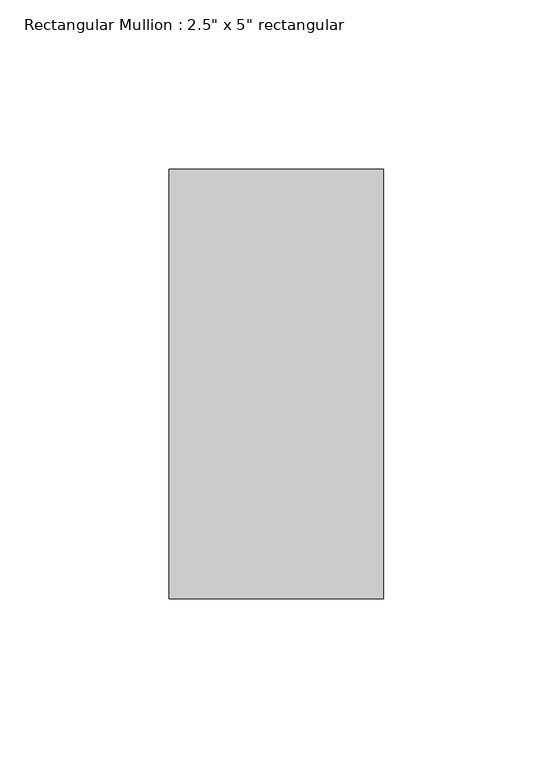
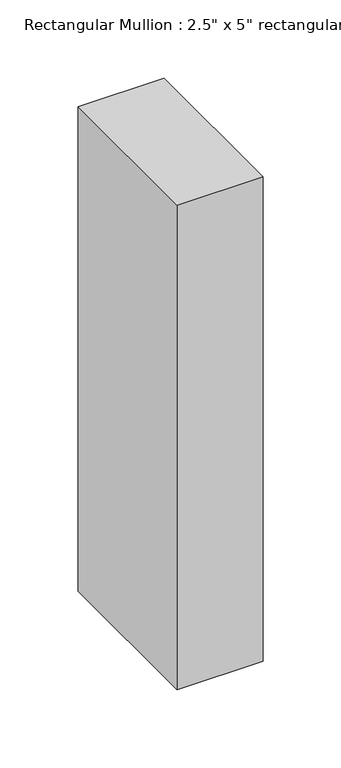
"""IFC4 building model written with IfcOpenShell, lengths in millimetres: member geometry."""

from ifc_helpers import new_model, si_unit, frame, origin, place, context, project, spatial, polyline, outline, extrude, source, transform, mapped, element, save


def member_e756d367(model_context):
    return source(origin(), model_context, "Body", "SweptSolid", [
        extrude(outline(polyline([(31.75, 63.5), (31.75, -63.5), (-31.75, -63.5), (-31.75, 63.5), (31.75, 63.5)])), frame((0.0, 0.0, -378.8833333), z_axis=(0.0, 0.0, 1.0), x_axis=(1.0, 0.0, 0.0)), (0.0, 0.0, 1.0), 378.8833333),
    ])


if __name__ == "__main__":
    model = new_model("IFC4")
    model_context = context("Model", 3, world=origin())
    ifc_project = project(units=[si_unit("LENGTHUNIT", "METRE", prefix="MILLI")], contexts=[model_context])
    site = spatial("IfcSite", under=ifc_project)
    building = spatial("IfcBuilding", under=site)
    placement = place(None, origin())
    member_shape = member_e756d367(model_context)
    element("IfcMember", 1, ObjectType="Rectangular Mullion : 2.5\" x 5\" rectangular", at=placement, inside=building, context=model_context, shape_type="MappedRepresentation", body=[
        mapped(member_shape, transform((0.0, 0.0, 0.0), x_axis=(1.0, 0.0, 0.0), y_axis=(0.0, 1.0, 0.0), z_axis=(0.0, 0.0, 1.0))),
    ])
    save(model, "model.ifc")

# Revit data of these elements
# Type "Rectangular Mullion : 2.5\" x 5\" rectangular"
#   built-in parameter 1007304 = 0.416667 (stored number, unit not read)
#   built-in parameter 1007301 = 0.104167 (stored number, unit not read)
#   built-in parameter 1007300 = 0.104167 (stored number, unit not read)
